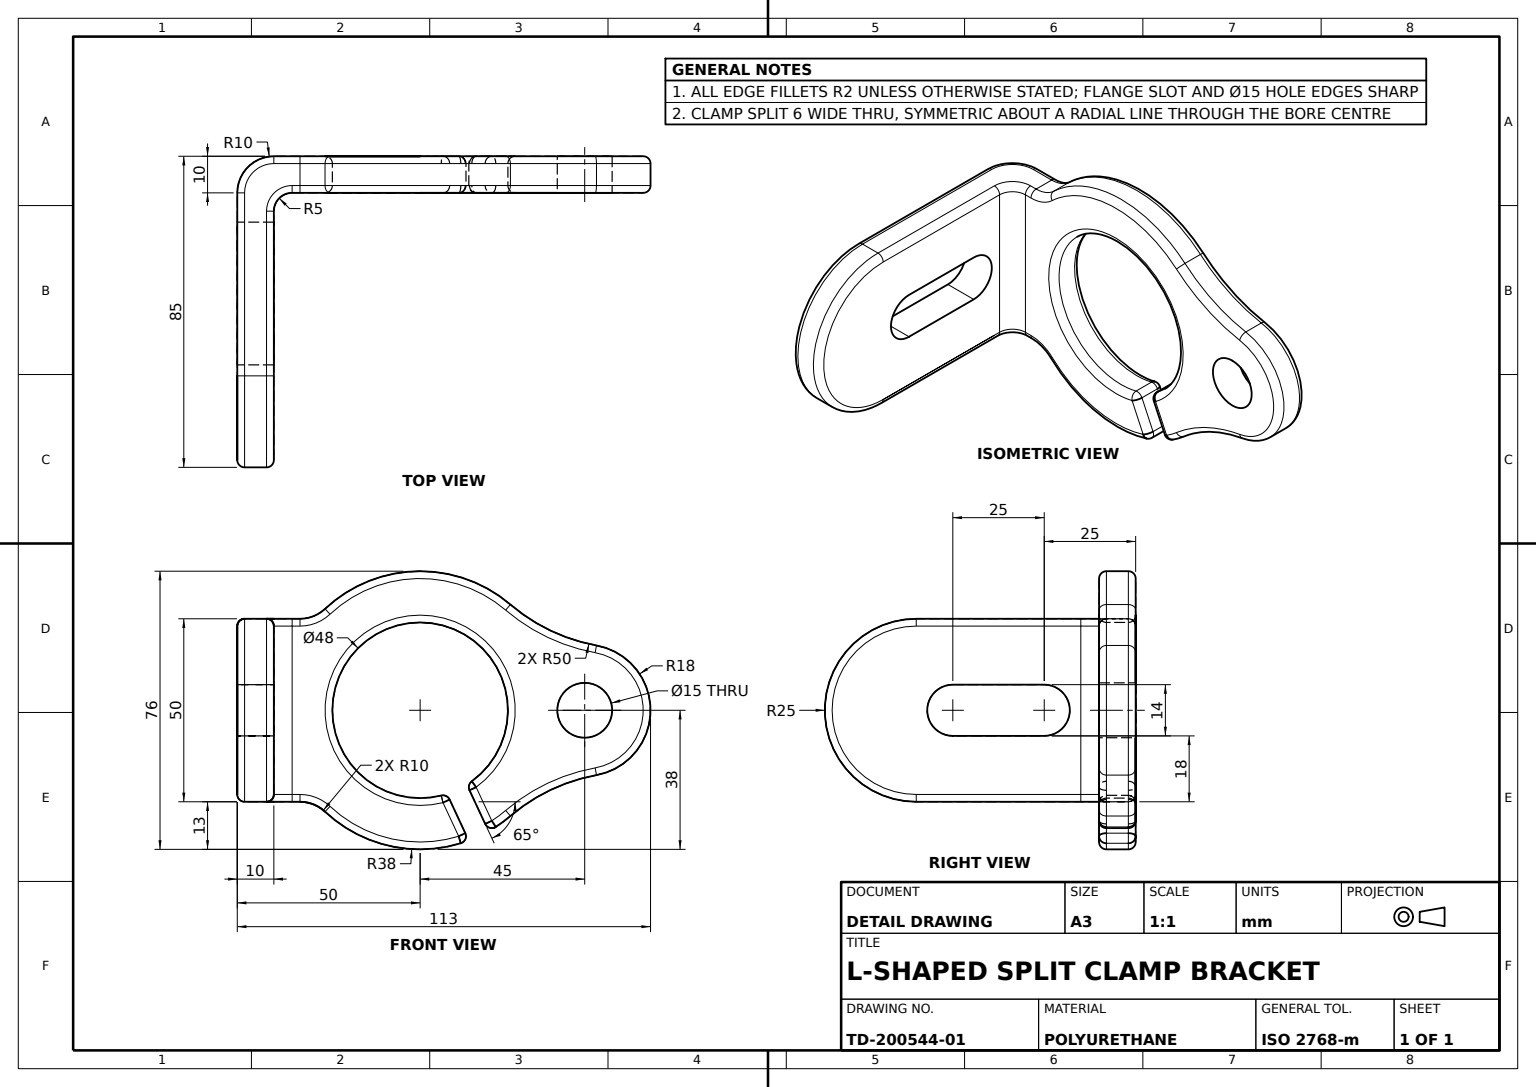
SolidWorks part; units mm, degrees
material "POLYURETHANE (11671)"
ref_plane "Front Plane" through (0, 0, 0) normal (0, 0, 1) x (1, 0, 0)
ref_plane "Top Plane" through (0, 0, 0) normal (0, 1, 0) x (1, 0, 0)
ref_plane "Right Plane" through (0, 0, 0) normal (1, 0, 0) x (0, 0, -1)
sketch "Clamp Plate Sketch" plane through (0, 0, 0) normal (0, 0, 1) x (1, 0, 0)
  line L0 (25, 0) -> (25, -17.1519)
  line L1 (25, 0) -> (-25, 0)
  line L2 (-25, 0) -> (-25, -17.1519)
  line L3 (0, 0) -> (0, -129.5929) construction
  circle A1 centre (0, -50) radius 24
  circle A2 centre (0, -95) radius 7.5
  arc A3 (-17.7095, -98.2206) -> (17.7095, -98.2206) centre (0, -95) ccw
  arc A4 (28.8898, -74.6856) -> (27.7083, -23.9952) centre (0, -50) ccw
  arc A5 (-17.7095, -98.2206) -> (-28.8898, -74.6856) centre (-66.9027, -107.1667) ccw
  arc A6 (17.7095, -98.2206) -> (28.8898, -74.6856) centre (66.9027, -107.1667) cw
  arc A7 (-27.7083, -23.9952) -> (-28.8898, -74.6856) centre (0, -50) ccw
  arc A8 (27.7083, -23.9952) -> (25, -17.1519) centre (35, -17.1519) cw
  arc A9 (-27.7083, -23.9952) -> (-25, -17.1519) centre (-35, -17.1519) ccw
  dimension "D2" = 15
  dimension "D4" = 48
  dimension "D5" = 50
  dimension "D6" = 36
  dimension "D7" = 50
  dimension "D9" = 10
  dimension "D10" = 38
  dimension "D1" = 50
  dimension "D3" = 45
  dimension "D8" = 50
extrude "Clamp Ring Plate" add sketch "Clamp Plate Sketch" along normal blind 10
sketch "Top Flange Sketch" plane through (0, 0, 0) normal (0, 1, 0) x (1, 0, 0)
  line L0 (-25, -10) -> (25, -10)
  line L1 (25, -10) -> (25, 50)
  line L3 (-25, 50) -> (-25, -10)
  line L4 (0, 40) -> (0, 15) construction
  line L5 (7, 40) -> (7, 15)
  line L6 (-7, 40) -> (-7, 15)
  line L7 (-25, -10) -> (-25, 0) construction
  line L8 (25, 0) -> (-25, 0) construction
  arc A0 (7, 40) -> (-7, 40) centre (0, 40) ccw
  arc A1 (-7, 15) -> (7, 15) centre (0, 15) ccw
  arc A2 (-25, 50) -> (25, 50) centre (0, 50) cw
  point P9 (0, 27.5)
  point P16 (0, -10)
  dimension "D3" = 7
  dimension "D4" = 60
  dimension "D1" = 25
  dimension "D2" = 50
extrude "Slotted Top Flange" add sketch "Top Flange Sketch" against normal blind 10
sketch "Clamp Split Sketch" plane through (0, 0, 0) normal (0, 0, -1) x (-1, 0, 0)
  line L0 (0, -50) -> (-59.8422, -50) construction
  line L1 (0, -50) -> (-54.4559, -75.3932) construction
  line L2 (-37.7441, -64.2902) -> (-18.548, -55.339)
  line L3 (-35.2084, -69.7281) -> (-16.0123, -60.7768)
  line L4 (-16.0123, -60.7768) -> (-18.548, -55.339)
  line L5 (-35.2084, -69.7281) -> (-37.7441, -64.2902)
  line L6 (25, -10) -> (25, -17.1519) construction
  dimension "D1" = 25
  dimension "D2" = 6
  dimension "D3" = 41.0123
  dimension "D4" = 60.2084
extrude "Clamp Split Cut" cut sketch "Clamp Split Sketch" against normal through all
fillet "Flange Bend Fillet R5" radius 5 1 edges at (0, -10, 0)
fillet "Plate Corner Fillet R10" radius 10 1 edges at (0, 0, 10)
fillet "Edge Break Fillets R2" radius 2 40 edges at (-25, -13.5759, 10) (-25.7017, -20.8318, 10) (-25, -2.9289, 7.0711) (-37.9897, -49.1146, 10) (-25, 0, -25) (-21.7397, -85.712, 10) (0, 0, -75) (0, -10, -75) (0, -113, 10) (25, 0, -25) (21.7397, -85.712, 10) (25, -2.9289, 7.0711) (21.7397, -85.712, 0) (31.12, -71.8071, 10) (0, -113, 0) (25, -13.5759, 10) (31.12, -71.8071, 0) (33.0643, -68.7283, 5) (26.6886, -65.7553, 10) (-21.7397, -85.712, 0) (25.7017, -20.8318, 10) (20.3129, -62.7822, 5) (26.6886, -65.7553, 0) (-21.7514, -39.8572, 10) (-37.9897, -49.1146, 0) (37.2561, -42.5178, 10) (29.2243, -60.3174, 10) (-21.7514, -39.8572, 0) (22.8486, -57.3444, 5) (-25.7017, -20.8318, 0) (35.6001, -63.2904, 5) (29.2243, -60.3174, 0) (-25, -16.0759, 0) (37.2561, -42.5178, 0) (-25, -11.4645, -1.4645) (25.7017, -20.8318, 0) (-25, -10, -27.5) (25, -16.0759, 0) (25, -11.4645, -1.4645) (25, -10, -27.5)
